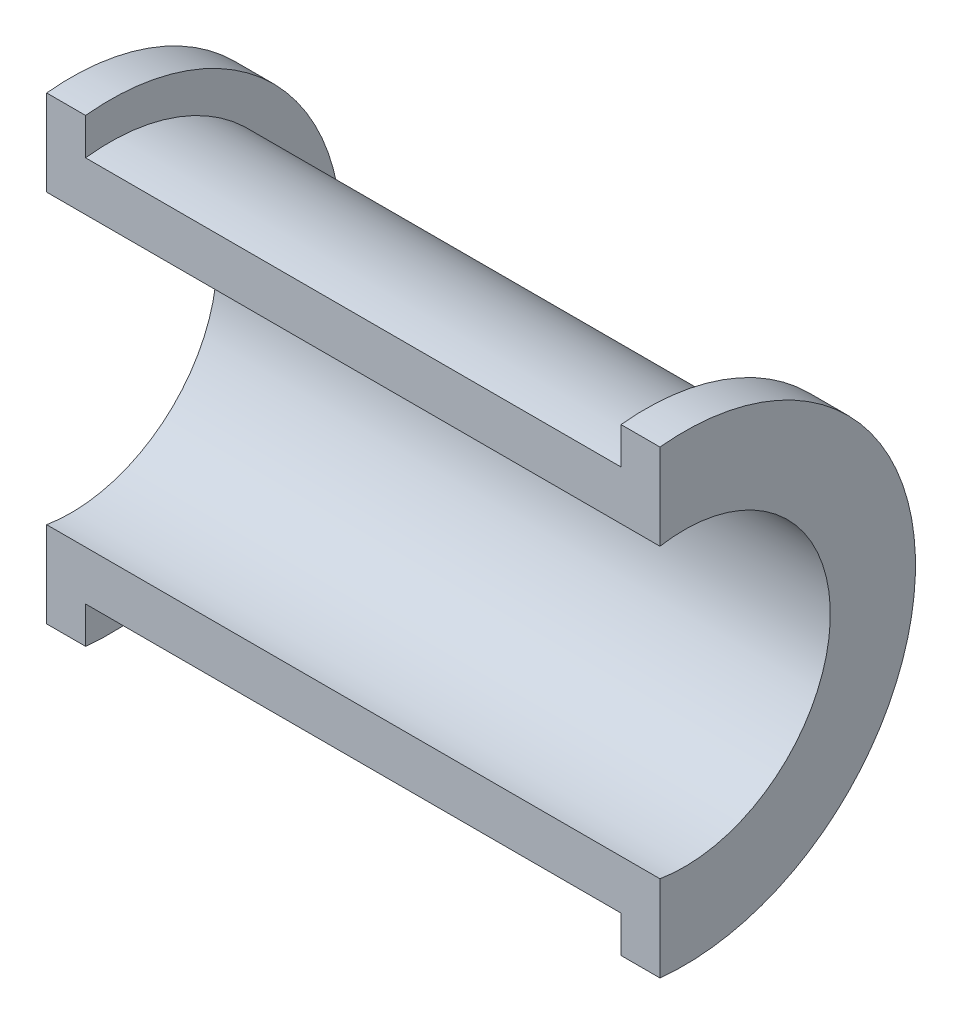
ISO-10303-21;
HEADER;
FILE_DESCRIPTION(('STEP AP214'),'2;1');
FILE_NAME('part.step','',(''),(''),'','','');
FILE_SCHEMA(('AUTOMOTIVE_DESIGN { 1 0 10303 214 1 1 1 1 }'));
ENDSEC;
DATA;
#1=APPLICATION_CONTEXT('core data for automotive mechanical design processes');
#2=APPLICATION_PROTOCOL_DEFINITION('international standard','automotive_design',2000,#1);
#3=PRODUCT_CONTEXT('',#1,'mechanical');
#4=PRODUCT('Part','Part','',(#3));
#5=PRODUCT_RELATED_PRODUCT_CATEGORY('part','',(#4));
#6=PRODUCT_DEFINITION_FORMATION('','',#4);
#7=PRODUCT_DEFINITION_CONTEXT('part definition',#1,'design');
#8=PRODUCT_DEFINITION('design','',#6,#7);
#9=PRODUCT_DEFINITION_SHAPE('','',#8);
#10=(LENGTH_UNIT() NAMED_UNIT(*) SI_UNIT(.MILLI.,.METRE.));
#11=(NAMED_UNIT(*) PLANE_ANGLE_UNIT() SI_UNIT($,.RADIAN.));
#12=(NAMED_UNIT(*) SI_UNIT($,.STERADIAN.) SOLID_ANGLE_UNIT());
#13=UNCERTAINTY_MEASURE_WITH_UNIT(LENGTH_MEASURE(1.E-05),#10,'distance_accuracy_value','');
#14=(GEOMETRIC_REPRESENTATION_CONTEXT(3) GLOBAL_UNCERTAINTY_ASSIGNED_CONTEXT((#13)) GLOBAL_UNIT_ASSIGNED_CONTEXT((#10,
#11,#12)) REPRESENTATION_CONTEXT('',''));
#15=CARTESIAN_POINT('',(0.,0.,0.));
#16=DIRECTION('',(0.,0.,1.));
#17=DIRECTION('',(1.,0.,0.));
#18=AXIS2_PLACEMENT_3D('',#15,#16,#17);
#19=CARTESIAN_POINT('',(55.,39.6862696659689,0.));
#20=DIRECTION('',(0.,0.,-1.));
#21=DIRECTION('',(-1.,0.,0.));
#22=AXIS2_PLACEMENT_3D('',#19,#20,#21);
#23=PLANE('',#22);
#24=DIRECTION('',(0.,1.,0.));
#25=VECTOR('',#24,1.);
#26=CARTESIAN_POINT('',(-63.,47.236109069228,-1.62031615845978E-13));
#27=LINE('',#26,#25);
#28=CARTESIAN_POINT('',(-63.,29.5803989154981,-1.01468133766529E-13));
#29=VERTEX_POINT('',#28);
#30=CARTESIAN_POINT('',(-63.,47.236109069228,-1.62031615845978E-13));
#31=VERTEX_POINT('',#30);
#32=EDGE_CURVE('E121',#29,#31,#27,.T.);
#33=ORIENTED_EDGE('',*,*,#32,.F.);
#34=DIRECTION('',(1.,0.,0.));
#35=VECTOR('',#34,1.);
#36=CARTESIAN_POINT('',(-100.,29.5803989154981,0.));
#37=LINE('',#36,#35);
#38=CARTESIAN_POINT('',(63.,29.5803989154981,0.));
#39=VERTEX_POINT('',#38);
#40=EDGE_CURVE('E54',#29,#39,#37,.T.);
#41=ORIENTED_EDGE('',*,*,#40,.T.);
#42=DIRECTION('',(0.,-1.,0.));
#43=VECTOR('',#42,1.);
#44=CARTESIAN_POINT('',(63.,47.236109069228,1.62031615845978E-13));
#45=LINE('',#44,#43);
#46=CARTESIAN_POINT('',(63.,47.236109069228,1.62031615845978E-13));
#47=VERTEX_POINT('',#46);
#48=EDGE_CURVE('E145',#47,#39,#45,.T.);
#49=ORIENTED_EDGE('',*,*,#48,.F.);
#50=DIRECTION('',(-1.,0.,0.));
#51=VECTOR('',#50,1.);
#52=CARTESIAN_POINT('',(63.,47.236109069228,1.62031615845978E-13));
#53=LINE('',#52,#51);
#54=CARTESIAN_POINT('',(55.,47.236109069228,1.62031615845978E-13));
#55=VERTEX_POINT('',#54);
#56=EDGE_CURVE('E154',#47,#55,#53,.T.);
#57=ORIENTED_EDGE('',*,*,#56,.T.);
#58=DIRECTION('',(0.,-1.,0.));
#59=VECTOR('',#58,1.);
#60=CARTESIAN_POINT('',(55.,47.236109069228,1.62031615845978E-13));
#61=LINE('',#60,#59);
#62=CARTESIAN_POINT('',(55.,39.6862696659688,1.361337867912E-13));
#63=VERTEX_POINT('',#62);
#64=EDGE_CURVE('E141',#55,#63,#61,.T.);
#65=ORIENTED_EDGE('',*,*,#64,.T.);
#66=DIRECTION('',(-1.,0.,0.));
#67=VECTOR('',#66,1.);
#68=CARTESIAN_POINT('',(55.,39.6862696659689,0.));
#69=LINE('',#68,#67);
#70=CARTESIAN_POINT('',(-55.,39.6862696659689,0.));
#71=VERTEX_POINT('',#70);
#72=EDGE_CURVE('E47',#63,#71,#69,.T.);
#73=ORIENTED_EDGE('',*,*,#72,.T.);
#74=DIRECTION('',(0.,1.,0.));
#75=VECTOR('',#74,1.);
#76=CARTESIAN_POINT('',(-55.,47.236109069228,-1.62031615845978E-13));
#77=LINE('',#76,#75);
#78=CARTESIAN_POINT('',(-55.,47.236109069228,-1.62031615845978E-13));
#79=VERTEX_POINT('',#78);
#80=EDGE_CURVE('E134',#71,#79,#77,.T.);
#81=ORIENTED_EDGE('',*,*,#80,.T.);
#82=DIRECTION('',(1.,0.,0.));
#83=VECTOR('',#82,1.);
#84=CARTESIAN_POINT('',(-63.,47.236109069228,-1.62031615845978E-13));
#85=LINE('',#84,#83);
#86=EDGE_CURVE('E125',#31,#79,#85,.T.);
#87=ORIENTED_EDGE('',*,*,#86,.F.);
#88=EDGE_LOOP('',(#33,#41,#49,#57,#65,#73,#81,#87));
#89=FACE_BOUND('',#88,.T.);
#90=ADVANCED_FACE('F41',(#89),#23,.F.);
#91=CARTESIAN_POINT('',(55.,0.,-5.));
#92=DIRECTION('',(-1.,0.,0.));
#93=DIRECTION('',(0.,0.,1.));
#94=AXIS2_PLACEMENT_3D('',#91,#92,#93);
#95=CYLINDRICAL_SURFACE('',#94,40.);
#96=CARTESIAN_POINT('',(-55.,0.,-5.));
#97=DIRECTION('',(1.,0.,0.));
#98=DIRECTION('',(0.,0.,-1.));
#99=AXIS2_PLACEMENT_3D('',#96,#97,#98);
#100=CIRCLE('',#99,40.);
#101=CARTESIAN_POINT('',(-55.,-39.6862696659688,1.361337867912E-13));
#102=VERTEX_POINT('',#101);
#103=EDGE_CURVE('E158',#102,#71,#100,.T.);
#104=ORIENTED_EDGE('',*,*,#103,.T.);
#105=ORIENTED_EDGE('',*,*,#72,.F.);
#106=CARTESIAN_POINT('',(55.,0.,-5.));
#107=DIRECTION('',(1.,0.,0.));
#108=DIRECTION('',(0.,0.,-1.));
#109=AXIS2_PLACEMENT_3D('',#106,#107,#108);
#110=CIRCLE('',#109,40.);
#111=CARTESIAN_POINT('',(55.,-39.6862696659689,0.));
#112=VERTEX_POINT('',#111);
#113=EDGE_CURVE('E157',#112,#63,#110,.T.);
#114=ORIENTED_EDGE('',*,*,#113,.F.);
#115=DIRECTION('',(-1.,0.,0.));
#116=VECTOR('',#115,1.);
#117=CARTESIAN_POINT('',(55.,-39.6862696659689,0.));
#118=LINE('',#117,#116);
#119=EDGE_CURVE('E64',#112,#102,#118,.T.);
#120=ORIENTED_EDGE('',*,*,#119,.T.);
#121=EDGE_LOOP('',(#104,#105,#114,#120));
#122=FACE_BOUND('',#121,.T.);
#123=ADVANCED_FACE('F43',(#122),#95,.T.);
#124=CARTESIAN_POINT('',(63.,-29.5803989154981,0.));
#125=VERTEX_POINT('',#124);
#126=CARTESIAN_POINT('',(63.,-47.236109069228,-1.62031615845978E-13));
#127=VERTEX_POINT('',#126);
#128=EDGE_CURVE('E118',#125,#127,#45,.T.);
#129=ORIENTED_EDGE('',*,*,#128,.F.);
#130=DIRECTION('',(1.,0.,0.));
#131=VECTOR('',#130,1.);
#132=CARTESIAN_POINT('',(-100.,-29.5803989154981,0.));
#133=LINE('',#132,#131);
#134=CARTESIAN_POINT('',(-63.,-29.5803989154981,1.01468133766529E-13));
#135=VERTEX_POINT('',#134);
#136=EDGE_CURVE('E104',#125,#135,#133,.F.);
#137=ORIENTED_EDGE('',*,*,#136,.T.);
#138=CARTESIAN_POINT('',(-63.,-47.236109069228,1.62031615845978E-13));
#139=VERTEX_POINT('',#138);
#140=EDGE_CURVE('E114',#139,#135,#27,.T.);
#141=ORIENTED_EDGE('',*,*,#140,.F.);
#142=DIRECTION('',(1.,0.,0.));
#143=VECTOR('',#142,1.);
#144=CARTESIAN_POINT('',(-63.,-47.236109069228,1.62031615845978E-13));
#145=LINE('',#144,#143);
#146=CARTESIAN_POINT('',(-55.,-47.236109069228,1.62031615845978E-13));
#147=VERTEX_POINT('',#146);
#148=EDGE_CURVE('E127',#139,#147,#145,.T.);
#149=ORIENTED_EDGE('',*,*,#148,.T.);
#150=EDGE_CURVE('E138',#147,#102,#77,.T.);
#151=ORIENTED_EDGE('',*,*,#150,.T.);
#152=ORIENTED_EDGE('',*,*,#119,.F.);
#153=CARTESIAN_POINT('',(55.,-47.236109069228,-1.62031615845978E-13));
#154=VERTEX_POINT('',#153);
#155=EDGE_CURVE('E147',#112,#154,#61,.T.);
#156=ORIENTED_EDGE('',*,*,#155,.T.);
#157=DIRECTION('',(-1.,0.,0.));
#158=VECTOR('',#157,1.);
#159=CARTESIAN_POINT('',(63.,-47.236109069228,-1.62031615845978E-13));
#160=LINE('',#159,#158);
#161=EDGE_CURVE('E150',#127,#154,#160,.T.);
#162=ORIENTED_EDGE('',*,*,#161,.F.);
#163=EDGE_LOOP('',(#129,#137,#141,#149,#151,#152,#156,#162));
#164=FACE_BOUND('',#163,.T.);
#165=ADVANCED_FACE('F112',(#164),#23,.F.);
#166=CARTESIAN_POINT('',(63.,0.,-5.));
#167=DIRECTION('',(-1.,0.,0.));
#168=DIRECTION('',(0.,0.,1.));
#169=AXIS2_PLACEMENT_3D('',#166,#167,#168);
#170=CYLINDRICAL_SURFACE('',#169,47.5);
#171=CARTESIAN_POINT('',(55.,0.,-5.));
#172=DIRECTION('',(1.,0.,0.));
#173=DIRECTION('',(0.,0.,-1.));
#174=AXIS2_PLACEMENT_3D('',#171,#172,#173);
#175=CIRCLE('',#174,47.5);
#176=EDGE_CURVE('E137',#154,#55,#175,.T.);
#177=ORIENTED_EDGE('',*,*,#176,.T.);
#178=ORIENTED_EDGE('',*,*,#56,.F.);
#179=CARTESIAN_POINT('',(63.,0.,-5.));
#180=DIRECTION('',(1.,0.,0.));
#181=DIRECTION('',(0.,0.,-1.));
#182=AXIS2_PLACEMENT_3D('',#179,#180,#181);
#183=CIRCLE('',#182,47.5);
#184=EDGE_CURVE('E139',#127,#47,#183,.T.);
#185=ORIENTED_EDGE('',*,*,#184,.F.);
#186=ORIENTED_EDGE('',*,*,#161,.T.);
#187=EDGE_LOOP('',(#177,#178,#185,#186));
#188=FACE_BOUND('',#187,.T.);
#189=ADVANCED_FACE('F177',(#188),#170,.T.);
#190=CARTESIAN_POINT('',(63.,0.,-5.));
#191=DIRECTION('',(1.,0.,0.));
#192=DIRECTION('',(0.,0.,-1.));
#193=AXIS2_PLACEMENT_3D('',#190,#191,#192);
#194=PLANE('',#193);
#195=CARTESIAN_POINT('',(63.,0.,-5.));
#196=DIRECTION('',(1.,0.,0.));
#197=DIRECTION('',(0.,0.,-1.));
#198=AXIS2_PLACEMENT_3D('',#195,#196,#197);
#199=CIRCLE('',#198,30.);
#200=EDGE_CURVE('E132',#125,#39,#199,.T.);
#201=ORIENTED_EDGE('',*,*,#200,.F.);
#202=ORIENTED_EDGE('',*,*,#128,.T.);
#203=ORIENTED_EDGE('',*,*,#184,.T.);
#204=ORIENTED_EDGE('',*,*,#48,.T.);
#205=EDGE_LOOP('',(#201,#202,#203,#204));
#206=FACE_BOUND('',#205,.T.);
#207=ADVANCED_FACE('F172',(#206),#194,.T.);
#208=CARTESIAN_POINT('',(55.,0.,-5.));
#209=DIRECTION('',(1.,0.,0.));
#210=DIRECTION('',(0.,0.,-1.));
#211=AXIS2_PLACEMENT_3D('',#208,#209,#210);
#212=PLANE('',#211);
#213=ORIENTED_EDGE('',*,*,#155,.F.);
#214=ORIENTED_EDGE('',*,*,#113,.T.);
#215=ORIENTED_EDGE('',*,*,#64,.F.);
#216=ORIENTED_EDGE('',*,*,#176,.F.);
#217=EDGE_LOOP('',(#213,#214,#215,#216));
#218=FACE_BOUND('',#217,.T.);
#219=ADVANCED_FACE('F181',(#218),#212,.F.);
#220=CARTESIAN_POINT('',(-63.,0.,-5.));
#221=DIRECTION('',(1.,0.,0.));
#222=DIRECTION('',(0.,0.,-1.));
#223=AXIS2_PLACEMENT_3D('',#220,#221,#222);
#224=CYLINDRICAL_SURFACE('',#223,47.5);
#225=CARTESIAN_POINT('',(-55.,0.,-5.));
#226=DIRECTION('',(-1.,0.,0.));
#227=DIRECTION('',(0.,0.,1.));
#228=AXIS2_PLACEMENT_3D('',#225,#226,#227);
#229=CIRCLE('',#228,47.5);
#230=EDGE_CURVE('E133',#79,#147,#229,.T.);
#231=ORIENTED_EDGE('',*,*,#230,.T.);
#232=ORIENTED_EDGE('',*,*,#148,.F.);
#233=CARTESIAN_POINT('',(-63.,0.,-5.));
#234=DIRECTION('',(-1.,0.,0.));
#235=DIRECTION('',(0.,0.,1.));
#236=AXIS2_PLACEMENT_3D('',#233,#234,#235);
#237=CIRCLE('',#236,47.5);
#238=EDGE_CURVE('E117',#31,#139,#237,.T.);
#239=ORIENTED_EDGE('',*,*,#238,.F.);
#240=ORIENTED_EDGE('',*,*,#86,.T.);
#241=EDGE_LOOP('',(#231,#232,#239,#240));
#242=FACE_BOUND('',#241,.T.);
#243=ADVANCED_FACE('F175',(#242),#224,.T.);
#244=CARTESIAN_POINT('',(-63.,0.,-5.));
#245=DIRECTION('',(-1.,0.,0.));
#246=DIRECTION('',(0.,0.,1.));
#247=AXIS2_PLACEMENT_3D('',#244,#245,#246);
#248=PLANE('',#247);
#249=CARTESIAN_POINT('',(-63.,0.,-5.));
#250=DIRECTION('',(-1.,0.,0.));
#251=DIRECTION('',(0.,0.,1.));
#252=AXIS2_PLACEMENT_3D('',#249,#250,#251);
#253=CIRCLE('',#252,30.);
#254=EDGE_CURVE('E11',#29,#135,#253,.T.);
#255=ORIENTED_EDGE('',*,*,#254,.F.);
#256=ORIENTED_EDGE('',*,*,#32,.T.);
#257=ORIENTED_EDGE('',*,*,#238,.T.);
#258=ORIENTED_EDGE('',*,*,#140,.T.);
#259=EDGE_LOOP('',(#255,#256,#257,#258));
#260=FACE_BOUND('',#259,.T.);
#261=ADVANCED_FACE('F116',(#260),#248,.T.);
#262=CARTESIAN_POINT('',(-55.,0.,-5.));
#263=DIRECTION('',(-1.,0.,0.));
#264=DIRECTION('',(0.,0.,1.));
#265=AXIS2_PLACEMENT_3D('',#262,#263,#264);
#266=PLANE('',#265);
#267=ORIENTED_EDGE('',*,*,#103,.F.);
#268=ORIENTED_EDGE('',*,*,#150,.F.);
#269=ORIENTED_EDGE('',*,*,#230,.F.);
#270=ORIENTED_EDGE('',*,*,#80,.F.);
#271=EDGE_LOOP('',(#267,#268,#269,#270));
#272=FACE_BOUND('',#271,.T.);
#273=ADVANCED_FACE('F166',(#272),#266,.F.);
#274=CARTESIAN_POINT('',(-100.,0.,-5.));
#275=DIRECTION('',(1.,0.,0.));
#276=DIRECTION('',(0.,0.,-1.));
#277=AXIS2_PLACEMENT_3D('',#274,#275,#276);
#278=CYLINDRICAL_SURFACE('',#277,30.);
#279=ORIENTED_EDGE('',*,*,#200,.T.);
#280=ORIENTED_EDGE('',*,*,#40,.F.);
#281=ORIENTED_EDGE('',*,*,#254,.T.);
#282=ORIENTED_EDGE('',*,*,#136,.F.);
#283=EDGE_LOOP('',(#279,#280,#281,#282));
#284=FACE_BOUND('',#283,.T.);
#285=ADVANCED_FACE('F102',(#284),#278,.F.);
#286=CLOSED_SHELL('',(#90,#123,#165,#189,#207,#219,#243,#261,#273,#285));
#287=MANIFOLD_SOLID_BREP('B2',#286);
#288=ADVANCED_BREP_SHAPE_REPRESENTATION('',(#18,#287),#14);
#289=SHAPE_DEFINITION_REPRESENTATION(#9,#288);
ENDSEC;
END-ISO-10303-21;
